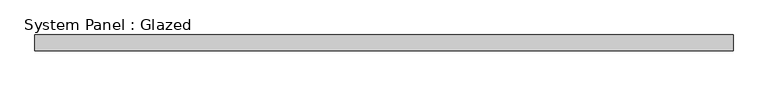
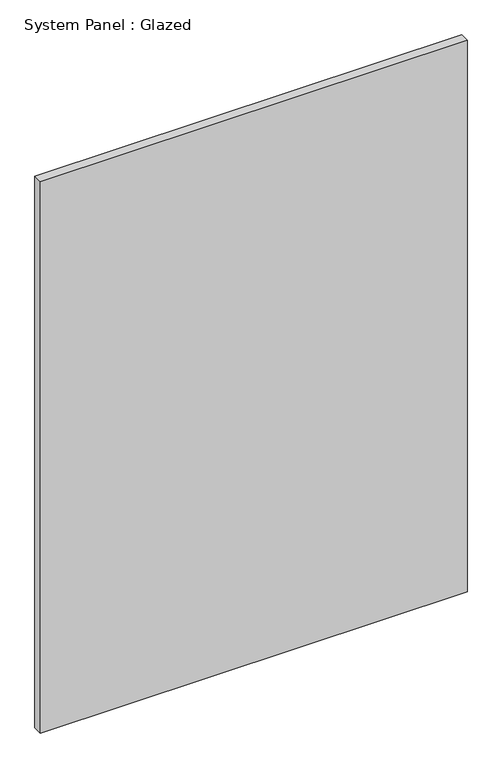
"""IFC4 building model written with IfcOpenShell, lengths in millimetres: plate geometry, System Panel : Glazed."""

from ifc_helpers import new_model, si_unit, origin, origin_with_axes, place, context, project, spatial, polyline, outline, extrude, source, transform, mapped, element, save


def system_panel_glazed_de05bfa4(model_context):
    return source(origin(), model_context, "Body", "SweptSolid", [
        extrude(outline(polyline([(561.975, 19.05), (-561.975, 19.05), (-561.975, 44.45), (561.975, 44.45), (561.975, 19.05)])), origin_with_axes(), (0.0, 0.0, 1.0), 1535.7829369),
    ])


if __name__ == "__main__":
    model = new_model("IFC4")
    model_context = context("Model", 3, world=origin())
    ifc_project = project(units=[si_unit("LENGTHUNIT", "METRE", prefix="MILLI")], contexts=[model_context])
    site = spatial("IfcSite", under=ifc_project)
    building = spatial("IfcBuilding", under=site)
    placement = place(None, origin())
    system_panel_glazed_shape = system_panel_glazed_de05bfa4(model_context)
    element("IfcPlate", 1, ObjectType="System Panel : Glazed", at=placement, inside=building, context=model_context, shape_type="MappedRepresentation", body=[
        mapped(system_panel_glazed_shape, transform((0.0, 0.0, 0.0), x_axis=(1.0, 0.0, 0.0), y_axis=(0.0, 1.0, 0.0), z_axis=(0.0, 0.0, 1.0))),
    ])
    save(model, "model.ifc")

# Revit data of these elements
# Type "System Panel : Glazed"
#   Construction Type Id = "GSP4R"
#   Analytic Construction = "1/8 in Pilkington single glazing"
#   Visual Light Transmittance = 0.9
#   Solar Heat Gain Coefficient = 0.86
#   Heat Transfer Coefficient (U) = 1.18115 BTU/(h·ft²·°F)
#   Define Thermal Properties by = 1
# Element 1 (IfcPlate, "System Panel : Glazed")
#   Materials on its faces: "Glass"
# Materials
#   "Glass": class "Glass", colour RGB 0 128 192, transparency 0.75, Description = "Soda Lime Glass", Cost = 0
